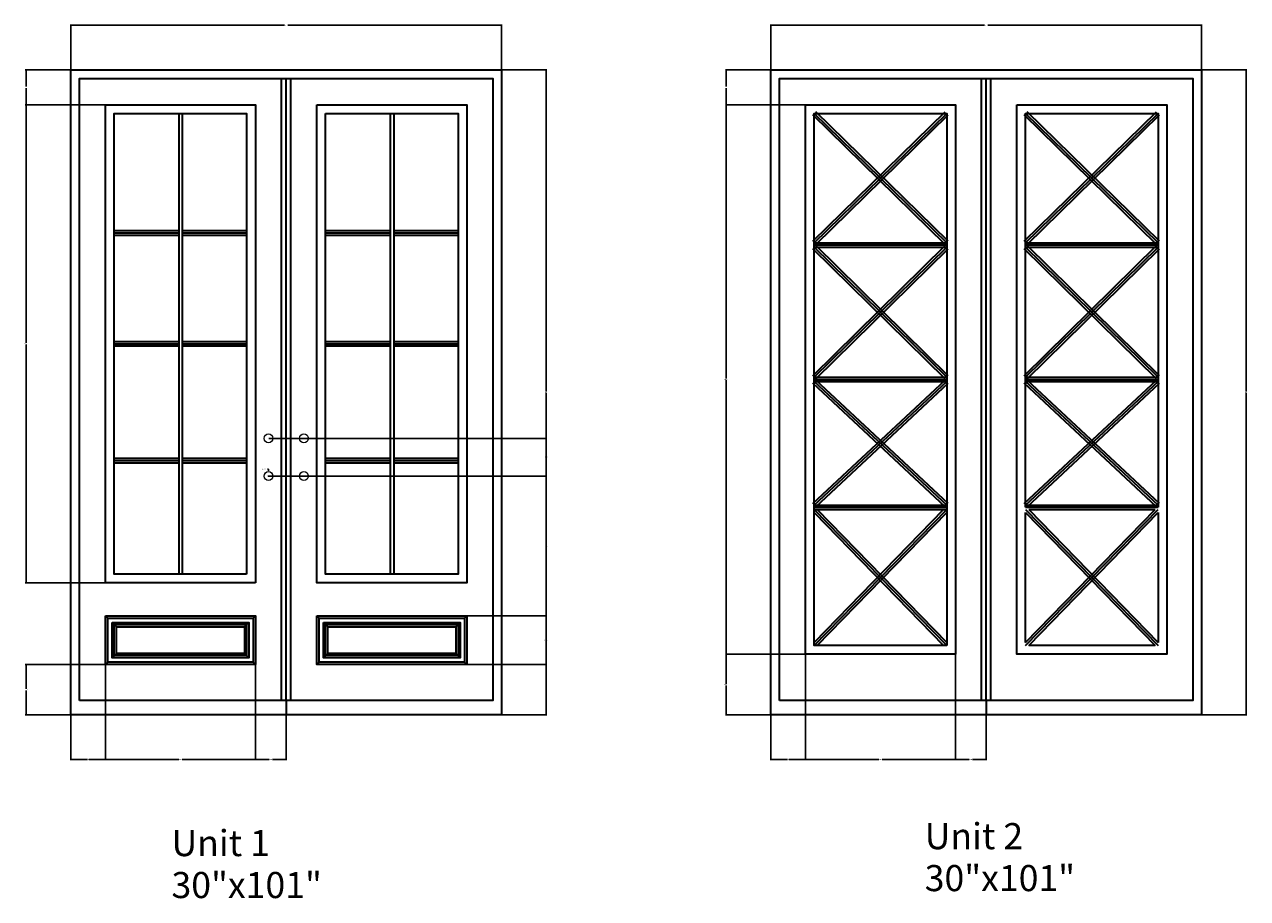
# Model space of a CAD drawing. Units: inches. Extents: x 1318 to 1980, y 617 to 1423.
# Tile 5 of 7: x 1351 to 1632, y 1222 to 1423. Entities that reach past the tile are written whole.
import ezdxf

# ---------------------------------------------------------------- set-up
doc = ezdxf.new("R2010")
doc.units = ezdxf.units.IN
doc.header["$MEASUREMENT"] = 0
for name, color, linetype, lineweight in [('A-ANNO-DIMS', 2, 'Continuous', 18), ('A-ANNO-TEXT', 7, 'Continuous', 25), ('A-DOOR', 4, 'Continuous', 35), ('A-DOOR-HDWR', 3, 'Continuous', 18)]:
    doc.layers.add(name, color=color, linetype=linetype, lineweight=lineweight)
doc.styles.get("Standard").update_dxf_attribs({"font": 'arial.ttf'})
doc.dimstyles.get("Standard").update_dxf_attribs({"dimtxt": 0.18, "dimasz": 0.18, "dimexe": 0.18, "dimexo": 0.0625, "dimgap": 0.09, "dimtad": 0, "dimtih": 1, "dimtoh": 1, "dimdec": 0, "dimzin": 0, "dimdsep": 46, "dimlunit": 3, "dimtxsty": 'Standard', "dimcen": 0.09, "dimadec": 0, "dimazin": 0, "dimtfac": 1, "dimtdec": 0, "dimtofl": 0, "dimtmove": 0, "dimatfit": 3, "dimfxl": 1, "dimtolj": 1, "dimtzin": 0, "dimarcsym": 0})

# ---------------------------------------------------------------- blocks, each defined once
blk = doc.blocks.new('DOOR-KNOB-SET')
for centre in [(1.01, 9.67), (9.16, 9.67), (1.01, 1.01), (9.16, 1.01)]:
    blk.add_circle(centre, 1.01)
blk = doc.blocks.new('*D4')
at = {"layer": 'A-ANNO-DIMS', "color": 0, "lineweight": -2, "transparency": 16777216}
for p, q in [((1453.13, 1287.17), (1471.5, 1287.17)), ((1471.32, 1286.99), (1471.32, 1281.77)), ((1471.32, 1276.2), (1471.32, 1281.41)), ((1453.13, 1276.02), (1471.5, 1276.02))]:
    blk.add_line(p, q, dxfattribs=at)
at = {"layer": 'A-ANNO-DIMS', "color": 0, "transparency": 16777216}
for points in [[(1471.29, 1286.99), (1471.35, 1286.99), (1471.32, 1287.17)], [(1471.29, 1276.2), (1471.35, 1276.2), (1471.32, 1276.02)]]:
    blk.add_solid(points, dxfattribs=at)
at = {"layer": 'Defpoints', "color": 0, "transparency": 16777216}
for p in [(1453.07, 1287.17), (1471.32, 1287.17), (1453.07, 1276.02)]:
    blk.add_point(p, dxfattribs=at)
at = {"layer": 'A-ANNO-DIMS', "color": 0, "transparency": 16777216, "insert": (1471.32, 1281.59), "char_height": 0.18, "attachment_point": 5}
blk.add_mtext('\\A1;11.142', dxfattribs=at)
blk = doc.blocks.new('*D5')
at = {"layer": 'A-ANNO-DIMS', "color": 0, "lineweight": -2, "transparency": 16777216}
for p, q in [((1407.58, 1319.29), (1471.5, 1319.29)), ((1471.32, 1319.11), (1471.32, 1303.41)), ((1471.32, 1287.35), (1471.32, 1303.04)), ((1453.13, 1287.17), (1471.5, 1287.17))]:
    blk.add_line(p, q, dxfattribs=at)
at = {"layer": 'A-ANNO-DIMS', "color": 0, "transparency": 16777216}
for points in [[(1471.29, 1319.11), (1471.35, 1319.11), (1471.32, 1319.29)], [(1471.29, 1287.35), (1471.35, 1287.35), (1471.32, 1287.17)]]:
    blk.add_solid(points, dxfattribs=at)
at = {"layer": 'Defpoints', "color": 0, "transparency": 16777216}
for p in [(1407.52, 1319.29), (1471.32, 1319.29), (1453.07, 1287.17)]:
    blk.add_point(p, dxfattribs=at)
at = {"layer": 'A-ANNO-DIMS', "color": 0, "transparency": 16777216, "insert": (1471.32, 1303.23), "char_height": 0.18, "attachment_point": 5}
blk.add_mtext('\\A1;32.12', dxfattribs=at)
blk = doc.blocks.new('*D6')
at = {"layer": 'A-ANNO-DIMS', "color": 0, "lineweight": -2, "transparency": 16777216}
for p, q in [((1407.58, 1327.95), (1471.5, 1327.95)), ((1471.32, 1327.77), (1471.32, 1323.8)), ((1471.32, 1319.47), (1471.32, 1323.44)), ((1407.58, 1319.29), (1471.5, 1319.29))]:
    blk.add_line(p, q, dxfattribs=at)
at = {"layer": 'A-ANNO-DIMS', "color": 0, "transparency": 16777216}
for points in [[(1471.29, 1327.77), (1471.35, 1327.77), (1471.32, 1327.95)], [(1471.29, 1319.47), (1471.35, 1319.47), (1471.32, 1319.29)]]:
    blk.add_solid(points, dxfattribs=at)
at = {"layer": 'Defpoints', "color": 0, "transparency": 16777216}
for p in [(1407.52, 1327.95), (1471.32, 1327.95), (1407.52, 1319.29)]:
    blk.add_point(p, dxfattribs=at)
at = {"layer": 'A-ANNO-DIMS', "color": 0, "transparency": 16777216, "insert": (1471.32, 1323.62), "char_height": 0.18, "attachment_point": 5}
blk.add_mtext('\\A1;8.663', dxfattribs=at)
blk = doc.blocks.new('*D7')
at = {"layer": 'A-ANNO-DIMS', "color": 0, "lineweight": -2, "transparency": 16777216}
for p, q in [((1362.09, 1412.68), (1362.09, 1423.04)), ((1362.27, 1422.86), (1411.18, 1422.86)), ((1460.89, 1422.86), (1411.97, 1422.86)), ((1461.07, 1412.68), (1461.07, 1423.04))]:
    blk.add_line(p, q, dxfattribs=at)
at = {"layer": 'A-ANNO-DIMS', "color": 0, "transparency": 16777216}
for points in [[(1362.27, 1422.89), (1362.27, 1422.83), (1362.09, 1422.86)], [(1460.89, 1422.89), (1460.89, 1422.83), (1461.07, 1422.86)]]:
    blk.add_solid(points, dxfattribs=at)
at = {"layer": 'Defpoints', "color": 0, "transparency": 16777216}
for p in [(1461.07, 1422.86), (1362.09, 1412.61), (1461.07, 1412.61)]:
    blk.add_point(p, dxfattribs=at)
at = {"layer": 'A-ANNO-DIMS', "color": 0, "transparency": 16777216, "insert": (1411.58, 1422.86), "char_height": 0.18, "attachment_point": 5}
blk.add_mtext('\\A1;98.98', dxfattribs=at)
blk = doc.blocks.new('*D8')
at = {"layer": 'A-ANNO-DIMS', "color": 0, "lineweight": -2, "transparency": 16777216}
for p, q in [((1461.13, 1412.61), (1471.5, 1412.61)), ((1471.32, 1412.43), (1471.32, 1338.7)), ((1471.32, 1264.59), (1471.32, 1338.33)), ((1461.13, 1264.41), (1471.5, 1264.41))]:
    blk.add_line(p, q, dxfattribs=at)
at = {"layer": 'A-ANNO-DIMS', "color": 0, "transparency": 16777216}
for points in [[(1471.29, 1412.43), (1471.35, 1412.43), (1471.32, 1412.61)], [(1471.29, 1264.59), (1471.35, 1264.59), (1471.32, 1264.41)]]:
    blk.add_solid(points, dxfattribs=at)
at = {"layer": 'Defpoints', "color": 0, "transparency": 16777216}
for p in [(1461.07, 1412.61), (1471.32, 1412.61), (1461.07, 1264.41)]:
    blk.add_point(p, dxfattribs=at)
at = {"layer": 'A-ANNO-DIMS', "color": 0, "transparency": 16777216, "insert": (1471.32, 1338.51), "char_height": 0.18, "attachment_point": 5}
blk.add_mtext('\\A1;148.2', dxfattribs=at)
blk = doc.blocks.new('*D9')
at = {"layer": 'A-ANNO-DIMS', "color": 0, "lineweight": -2, "transparency": 16777216}
for p, q in [((1370.09, 1275.96), (1370.09, 1253.98)), ((1362.09, 1264.35), (1362.09, 1253.98)), ((1362.27, 1254.16), (1365.94, 1254.16)), ((1369.91, 1254.16), (1366.24, 1254.16))]:
    blk.add_line(p, q, dxfattribs=at)
at = {"layer": 'A-ANNO-DIMS', "color": 0, "transparency": 16777216}
for points in [[(1362.27, 1254.19), (1362.27, 1254.13), (1362.09, 1254.16)], [(1369.91, 1254.19), (1369.91, 1254.13), (1370.09, 1254.16)]]:
    blk.add_solid(points, dxfattribs=at)
at = {"layer": 'Defpoints', "color": 0, "transparency": 16777216}
for p in [(1370.09, 1276.02), (1362.09, 1264.41), (1370.09, 1254.16)]:
    blk.add_point(p, dxfattribs=at)
at = {"layer": 'A-ANNO-DIMS', "color": 0, "transparency": 16777216, "insert": (1366.09, 1254.16), "char_height": 0.18, "attachment_point": 5}
blk.add_mtext('\\A1;8', dxfattribs=at)
blk = doc.blocks.new('*D10')
at = {"layer": 'A-ANNO-DIMS', "color": 0, "lineweight": -2, "transparency": 16777216}
for p, q in [((1370.09, 1275.96), (1370.09, 1253.98)), ((1404.51, 1275.96), (1404.51, 1253.98)), ((1370.27, 1254.16), (1386.91, 1254.16)), ((1404.33, 1254.16), (1387.69, 1254.16))]:
    blk.add_line(p, q, dxfattribs=at)
at = {"layer": 'A-ANNO-DIMS', "color": 0, "transparency": 16777216}
for points in [[(1370.27, 1254.19), (1370.27, 1254.13), (1370.09, 1254.16)], [(1404.33, 1254.19), (1404.33, 1254.13), (1404.51, 1254.16)]]:
    blk.add_solid(points, dxfattribs=at)
at = {"layer": 'Defpoints', "color": 0, "transparency": 16777216}
for p in [(1370.09, 1276.02), (1404.51, 1276.02), (1404.51, 1254.16)]:
    blk.add_point(p, dxfattribs=at)
at = {"layer": 'A-ANNO-DIMS', "color": 0, "transparency": 16777216, "insert": (1387.3, 1254.16), "char_height": 0.18, "attachment_point": 5}
blk.add_mtext('\\A1;34.42', dxfattribs=at)
blk = doc.blocks.new('*D11')
at = {"layer": 'A-ANNO-DIMS', "color": 0, "lineweight": -2, "transparency": 16777216}
for p, q in [((1404.51, 1275.96), (1404.51, 1253.98)), ((1411.58, 1264.35), (1411.58, 1253.98)), ((1404.69, 1254.16), (1407.65, 1254.16)), ((1411.4, 1254.16), (1408.44, 1254.16))]:
    blk.add_line(p, q, dxfattribs=at)
at = {"layer": 'A-ANNO-DIMS', "color": 0, "transparency": 16777216}
for points in [[(1404.69, 1254.19), (1404.69, 1254.13), (1404.51, 1254.16)], [(1411.4, 1254.19), (1411.4, 1254.13), (1411.58, 1254.16)]]:
    blk.add_solid(points, dxfattribs=at)
at = {"layer": 'Defpoints', "color": 0, "transparency": 16777216}
for p in [(1404.51, 1276.02), (1411.58, 1264.41), (1411.58, 1254.16)]:
    blk.add_point(p, dxfattribs=at)
at = {"layer": 'A-ANNO-DIMS', "color": 0, "transparency": 16777216, "insert": (1408.04, 1254.16), "char_height": 0.18, "attachment_point": 5}
blk.add_mtext('\\A1;7.068', dxfattribs=at)
blk = doc.blocks.new('*D12')
at = {"layer": 'A-ANNO-DIMS', "color": 0, "lineweight": -2, "transparency": 16777216}
for p, q in [((1370.02, 1276.02), (1351.66, 1276.02)), ((1351.84, 1275.84), (1351.84, 1270.4)), ((1351.84, 1264.59), (1351.84, 1270.04)), ((1362.02, 1264.41), (1351.66, 1264.41))]:
    blk.add_line(p, q, dxfattribs=at)
at = {"layer": 'A-ANNO-DIMS', "color": 0, "transparency": 16777216}
for points in [[(1351.81, 1275.84), (1351.87, 1275.84), (1351.84, 1276.02)], [(1351.81, 1264.59), (1351.87, 1264.59), (1351.84, 1264.41)]]:
    blk.add_solid(points, dxfattribs=at)
at = {"layer": 'Defpoints', "color": 0, "transparency": 16777216}
for p in [(1351.84, 1276.02), (1370.09, 1276.02), (1362.09, 1264.41)]:
    blk.add_point(p, dxfattribs=at)
at = {"layer": 'A-ANNO-DIMS', "color": 0, "transparency": 16777216, "insert": (1351.84, 1270.22), "char_height": 0.18, "attachment_point": 5}
blk.add_mtext('\\A1;11.61', dxfattribs=at)
blk = doc.blocks.new('*D13')
at = {"layer": 'A-ANNO-DIMS', "color": 0, "lineweight": -2, "transparency": 16777216}
for p, q in [((1370.02, 1404.61), (1351.66, 1404.61)), ((1351.84, 1404.43), (1351.84, 1349.86)), ((1351.84, 1294.93), (1351.84, 1349.5)), ((1370.02, 1294.75), (1351.66, 1294.75))]:
    blk.add_line(p, q, dxfattribs=at)
at = {"layer": 'A-ANNO-DIMS', "color": 0, "transparency": 16777216}
for points in [[(1351.81, 1404.43), (1351.87, 1404.43), (1351.84, 1404.61)], [(1351.81, 1294.93), (1351.87, 1294.93), (1351.84, 1294.75)]]:
    blk.add_solid(points, dxfattribs=at)
at = {"layer": 'Defpoints', "color": 0, "transparency": 16777216}
for p in [(1351.84, 1404.61), (1370.09, 1404.61), (1370.09, 1294.75)]:
    blk.add_point(p, dxfattribs=at)
at = {"layer": 'A-ANNO-DIMS', "color": 0, "transparency": 16777216, "insert": (1351.84, 1349.68), "char_height": 0.18, "attachment_point": 5}
blk.add_mtext('\\A1;109.87', dxfattribs=at)
blk = doc.blocks.new('*D14')
at = {"layer": 'A-ANNO-DIMS', "color": 0, "lineweight": -2, "transparency": 16777216}
for p, q in [((1362.02, 1412.61), (1351.66, 1412.61)), ((1351.84, 1412.43), (1351.84, 1408.8)), ((1351.84, 1404.79), (1351.84, 1408.43)), ((1370.02, 1404.61), (1351.66, 1404.61))]:
    blk.add_line(p, q, dxfattribs=at)
at = {"layer": 'A-ANNO-DIMS', "color": 0, "transparency": 16777216}
for points in [[(1351.81, 1412.43), (1351.87, 1412.43), (1351.84, 1412.61)], [(1351.81, 1404.79), (1351.87, 1404.79), (1351.84, 1404.61)]]:
    blk.add_solid(points, dxfattribs=at)
at = {"layer": 'Defpoints', "color": 0, "transparency": 16777216}
for p in [(1351.84, 1412.61), (1362.09, 1412.61), (1370.09, 1404.61)]:
    blk.add_point(p, dxfattribs=at)
at = {"layer": 'A-ANNO-DIMS', "color": 0, "transparency": 16777216, "insert": (1351.84, 1408.61), "char_height": 0.18, "attachment_point": 5}
blk.add_mtext('\\A1;8', dxfattribs=at)
blk = doc.blocks.new('*D15')
at = {"layer": 'A-ANNO-DIMS', "color": 0, "lineweight": -2, "transparency": 16777216}
for p, q in [((1522.91, 1412.68), (1522.91, 1423.04)), ((1523.09, 1422.86), (1572, 1422.86)), ((1621.7, 1422.86), (1572.79, 1422.86)), ((1621.88, 1412.68), (1621.88, 1423.04))]:
    blk.add_line(p, q, dxfattribs=at)
at = {"layer": 'A-ANNO-DIMS', "color": 0, "transparency": 16777216}
for points in [[(1523.09, 1422.89), (1523.09, 1422.83), (1522.91, 1422.86)], [(1621.7, 1422.89), (1621.7, 1422.83), (1621.88, 1422.86)]]:
    blk.add_solid(points, dxfattribs=at)
at = {"layer": 'Defpoints', "color": 0, "transparency": 16777216}
for p in [(1621.88, 1422.86), (1522.91, 1412.61), (1621.88, 1412.61)]:
    blk.add_point(p, dxfattribs=at)
at = {"layer": 'A-ANNO-DIMS', "color": 0, "transparency": 16777216, "insert": (1572.39, 1422.86), "char_height": 0.18, "attachment_point": 5}
blk.add_mtext('\\A1;98.98', dxfattribs=at)
blk = doc.blocks.new('*D16')
at = {"layer": 'A-ANNO-DIMS', "color": 0, "lineweight": -2, "transparency": 16777216}
for p, q in [((1621.95, 1412.61), (1632.31, 1412.61)), ((1632.13, 1412.43), (1632.13, 1338.7)), ((1632.13, 1264.59), (1632.13, 1338.33)), ((1621.95, 1264.41), (1632.31, 1264.41))]:
    blk.add_line(p, q, dxfattribs=at)
at = {"layer": 'A-ANNO-DIMS', "color": 0, "transparency": 16777216}
for points in [[(1632.1, 1412.43), (1632.16, 1412.43), (1632.13, 1412.61)], [(1632.1, 1264.59), (1632.16, 1264.59), (1632.13, 1264.41)]]:
    blk.add_solid(points, dxfattribs=at)
at = {"layer": 'Defpoints', "color": 0, "transparency": 16777216}
for p in [(1621.88, 1412.61), (1632.13, 1412.61), (1621.88, 1264.41)]:
    blk.add_point(p, dxfattribs=at)
at = {"layer": 'A-ANNO-DIMS', "color": 0, "transparency": 16777216, "insert": (1632.13, 1338.51), "char_height": 0.18, "attachment_point": 5}
blk.add_mtext('\\A1;148.2', dxfattribs=at)
blk = doc.blocks.new('*D17')
at = {"layer": 'A-ANNO-DIMS', "color": 0, "lineweight": -2, "transparency": 16777216}
for p, q in [((1530.91, 1278.29), (1530.91, 1253.98)), ((1522.91, 1264.35), (1522.91, 1253.98)), ((1523.09, 1254.16), (1526.76, 1254.16)), ((1530.73, 1254.16), (1527.05, 1254.16))]:
    blk.add_line(p, q, dxfattribs=at)
at = {"layer": 'A-ANNO-DIMS', "color": 0, "transparency": 16777216}
for points in [[(1523.09, 1254.19), (1523.09, 1254.13), (1522.91, 1254.16)], [(1530.73, 1254.19), (1530.73, 1254.13), (1530.91, 1254.16)]]:
    blk.add_solid(points, dxfattribs=at)
at = {"layer": 'Defpoints', "color": 0, "transparency": 16777216}
for p in [(1530.91, 1278.35), (1522.91, 1264.41), (1530.91, 1254.16)]:
    blk.add_point(p, dxfattribs=at)
at = {"layer": 'A-ANNO-DIMS', "color": 0, "transparency": 16777216, "insert": (1526.91, 1254.16), "char_height": 0.18, "attachment_point": 5}
blk.add_mtext('\\A1;8', dxfattribs=at)
blk = doc.blocks.new('*D18')
at = {"layer": 'A-ANNO-DIMS', "color": 0, "lineweight": -2, "transparency": 16777216}
for p, q in [((1530.91, 1278.29), (1530.91, 1253.98)), ((1565.33, 1278.29), (1565.33, 1253.98)), ((1531.09, 1254.16), (1547.72, 1254.16)), ((1565.15, 1254.16), (1548.51, 1254.16))]:
    blk.add_line(p, q, dxfattribs=at)
at = {"layer": 'A-ANNO-DIMS', "color": 0, "transparency": 16777216}
for points in [[(1531.09, 1254.19), (1531.09, 1254.13), (1530.91, 1254.16)], [(1565.15, 1254.19), (1565.15, 1254.13), (1565.33, 1254.16)]]:
    blk.add_solid(points, dxfattribs=at)
at = {"layer": 'Defpoints', "color": 0, "transparency": 16777216}
for p in [(1530.91, 1278.35), (1565.33, 1278.35), (1565.33, 1254.16)]:
    blk.add_point(p, dxfattribs=at)
at = {"layer": 'A-ANNO-DIMS', "color": 0, "transparency": 16777216, "insert": (1548.12, 1254.16), "char_height": 0.18, "attachment_point": 5}
blk.add_mtext('\\A1;34.42', dxfattribs=at)
blk = doc.blocks.new('*D19')
at = {"layer": 'A-ANNO-DIMS', "color": 0, "lineweight": -2, "transparency": 16777216}
for p, q in [((1565.33, 1278.29), (1565.33, 1253.98)), ((1572.39, 1264.35), (1572.39, 1253.98)), ((1565.51, 1254.16), (1568.47, 1254.16)), ((1572.21, 1254.16), (1569.25, 1254.16))]:
    blk.add_line(p, q, dxfattribs=at)
at = {"layer": 'A-ANNO-DIMS', "color": 0, "transparency": 16777216}
for points in [[(1565.51, 1254.19), (1565.51, 1254.13), (1565.33, 1254.16)], [(1572.21, 1254.19), (1572.21, 1254.13), (1572.39, 1254.16)]]:
    blk.add_solid(points, dxfattribs=at)
at = {"layer": 'Defpoints', "color": 0, "transparency": 16777216}
for p in [(1565.33, 1278.35), (1572.39, 1264.41), (1572.39, 1254.16)]:
    blk.add_point(p, dxfattribs=at)
at = {"layer": 'A-ANNO-DIMS', "color": 0, "transparency": 16777216, "insert": (1568.86, 1254.16), "char_height": 0.18, "attachment_point": 5}
blk.add_mtext('\\A1;7.068', dxfattribs=at)
blk = doc.blocks.new('*D20')
at = {"layer": 'A-ANNO-DIMS', "color": 0, "lineweight": -2, "transparency": 16777216}
for p, q in [((1530.84, 1278.35), (1512.48, 1278.35)), ((1512.66, 1278.17), (1512.66, 1271.56)), ((1512.66, 1264.59), (1512.66, 1271.2)), ((1522.84, 1264.41), (1512.48, 1264.41))]:
    blk.add_line(p, q, dxfattribs=at)
at = {"layer": 'A-ANNO-DIMS', "color": 0, "transparency": 16777216}
for points in [[(1512.63, 1278.17), (1512.69, 1278.17), (1512.66, 1278.35)], [(1512.63, 1264.59), (1512.69, 1264.59), (1512.66, 1264.41)]]:
    blk.add_solid(points, dxfattribs=at)
at = {"layer": 'Defpoints', "color": 0, "transparency": 16777216}
for p in [(1512.66, 1278.35), (1530.91, 1278.35), (1522.91, 1264.41)]:
    blk.add_point(p, dxfattribs=at)
at = {"layer": 'A-ANNO-DIMS', "color": 0, "transparency": 16777216, "insert": (1512.66, 1271.38), "char_height": 0.18, "attachment_point": 5}
blk.add_mtext('\\A1;13.939', dxfattribs=at)
blk = doc.blocks.new('*D21')
at = {"layer": 'A-ANNO-DIMS', "color": 0, "lineweight": -2, "transparency": 16777216}
for p, q in [((1530.84, 1404.61), (1512.48, 1404.61)), ((1512.66, 1404.43), (1512.66, 1341.67)), ((1512.66, 1278.53), (1512.66, 1341.3)), ((1530.84, 1278.35), (1512.48, 1278.35))]:
    blk.add_line(p, q, dxfattribs=at)
at = {"layer": 'A-ANNO-DIMS', "color": 0, "transparency": 16777216}
for points in [[(1512.63, 1404.43), (1512.69, 1404.43), (1512.66, 1404.61)], [(1512.63, 1278.53), (1512.69, 1278.53), (1512.66, 1278.35)]]:
    blk.add_solid(points, dxfattribs=at)
at = {"layer": 'Defpoints', "color": 0, "transparency": 16777216}
for p in [(1512.66, 1404.61), (1530.91, 1404.61), (1530.91, 1278.35)]:
    blk.add_point(p, dxfattribs=at)
at = {"layer": 'A-ANNO-DIMS', "color": 0, "transparency": 16777216, "insert": (1512.66, 1341.48), "char_height": 0.18, "attachment_point": 5}
blk.add_mtext('\\A1;126.26', dxfattribs=at)
blk = doc.blocks.new('*D22')
at = {"layer": 'A-ANNO-DIMS', "color": 0, "lineweight": -2, "transparency": 16777216}
for p, q in [((1522.84, 1412.61), (1512.48, 1412.61)), ((1512.66, 1412.43), (1512.66, 1408.8)), ((1512.66, 1404.79), (1512.66, 1408.43)), ((1530.84, 1404.61), (1512.48, 1404.61))]:
    blk.add_line(p, q, dxfattribs=at)
at = {"layer": 'A-ANNO-DIMS', "color": 0, "transparency": 16777216}
for points in [[(1512.63, 1412.43), (1512.69, 1412.43), (1512.66, 1412.61)], [(1512.63, 1404.79), (1512.69, 1404.79), (1512.66, 1404.61)]]:
    blk.add_solid(points, dxfattribs=at)
at = {"layer": 'Defpoints', "color": 0, "transparency": 16777216}
for p in [(1512.66, 1412.61), (1522.91, 1412.61), (1530.91, 1404.61)]:
    blk.add_point(p, dxfattribs=at)
at = {"layer": 'A-ANNO-DIMS', "color": 0, "transparency": 16777216, "insert": (1512.66, 1408.61), "char_height": 0.18, "attachment_point": 5}
blk.add_mtext('\\A1;8', dxfattribs=at)
blk = doc.blocks.new('*D104')
at = {"layer": 'A-ANNO-DIMS', "color": 0, "lineweight": -2, "transparency": 16777216}
for p, q in [((1407.31, 1320.9), (1407.49, 1320.9)), ((1407.49, 1320.9), (1407.5, 1320.47)), ((1407.43, 1319.29), (1407.61, 1319.29)), ((1407.52, 1319.2), (1407.52, 1319.38))]:
    blk.add_line(p, q, dxfattribs=at)
at = {"layer": 'A-ANNO-DIMS', "color": 0, "transparency": 16777216}
blk.add_solid([(1407.53, 1320.48), (1407.47, 1320.47), (1407.5, 1320.29)], dxfattribs=at)
at = {"layer": 'Defpoints', "color": 0, "transparency": 16777216}
for p in [(1407.5, 1320.29), (1407.53, 1318.28)]:
    blk.add_point(p, dxfattribs=at)
at = {"layer": 'A-ANNO-DIMS', "color": 0, "transparency": 16777216, "insert": (1406.63, 1320.9), "char_height": 0.18, "attachment_point": 5}
blk.add_mtext('\\A1;4X ∅2.017', dxfattribs=at)

msp = doc.modelspace()

# ---------------------------------------------------------------- linework, layer by layer
at = {"layer": 'A-DOOR'}
for p, q in [((1410.5087, 1267.7069), (1410.5087, 1410.615)), ((1411.5767, 1267.7069), (1411.5767, 1410.615)), ((1412.6446, 1267.7069), (1412.6446, 1410.615)), ((1571.3268, 1267.7069), (1571.3268, 1410.615)), ((1572.3947, 1267.7069), (1572.3947, 1410.615)), ((1573.4627, 1267.7069), (1573.4627, 1410.615)), ((1386.9042, 1402.615), (1386.9042, 1296.7497)), ((1387.7277, 1402.615), (1387.7277, 1296.7497)), ((1435.4614, 1402.615), (1435.4614, 1296.7497)), ((1436.2849, 1402.615), (1436.2849, 1296.7497)), ((1532.556, 1373.2363), (1562.9773, 1402.9725)), ((1562.9773, 1372.5212), (1532.556, 1402.2574)), ((1532.9055, 1372.8787), (1563.3268, 1402.615)), ((1563.3268, 1372.8787), (1532.9055, 1402.615)), ((1563.6763, 1373.2363), (1533.255, 1402.9725)), ((1533.255, 1372.5212), (1563.6763, 1402.2574)), ((1581.1132, 1373.2363), (1611.5345, 1402.9725)), ((1611.5345, 1372.5212), (1581.1132, 1402.2574)), ((1581.4627, 1372.8787), (1611.884, 1402.615)), ((1611.884, 1372.8787), (1581.4627, 1402.615)), ((1612.2335, 1373.2363), (1581.8122, 1402.9725)), ((1581.8122, 1372.5212), (1612.2335, 1402.2574)), ((1372.0874, 1375.6684), (1386.9042, 1375.6684)), ((1372.0874, 1375.1684), (1386.9042, 1375.1684)), ((1372.0874, 1374.6684), (1386.9042, 1374.6684)), ((1387.7277, 1375.6684), (1402.5087, 1375.6684)), ((1387.7277, 1375.1684), (1402.5087, 1375.1684)), ((1387.7277, 1374.6684), (1402.5087, 1374.6684)), ((1420.6446, 1375.6684), (1435.4614, 1375.6684)), ((1420.6446, 1375.1684), (1435.4614, 1375.1684)), ((1420.6446, 1374.6684), (1435.4614, 1374.6684)), ((1436.2849, 1375.6684), (1451.0659, 1375.6684)), ((1436.2849, 1375.1684), (1451.0659, 1375.1684)), ((1436.2849, 1374.6684), (1451.0659, 1374.6684)), ((1532.555, 1342.3402), (1562.9763, 1372.2354)), ((1562.9763, 1341.6269), (1532.555, 1371.5221)), ((1532.9055, 1372.8787), (1563.3268, 1372.8787)), ((1532.9055, 1372.3787), (1563.3268, 1372.3787)), ((1532.9055, 1371.8787), (1563.3268, 1371.8787)), ((1532.9055, 1341.9835), (1563.3268, 1371.8787)), ((1563.3268, 1341.9835), (1532.9055, 1371.8787)), ((1563.6772, 1342.3402), (1533.256, 1372.2354)), ((1533.256, 1341.6269), (1563.6772, 1371.5221)), ((1581.1122, 1342.3402), (1611.5335, 1372.2354)), ((1611.5335, 1341.6269), (1581.1122, 1371.5221)), ((1581.4627, 1372.8787), (1611.884, 1372.8787)), ((1581.4627, 1372.3787), (1611.884, 1372.3787)), ((1581.4627, 1371.8787), (1611.884, 1371.8787)), ((1581.4627, 1341.9835), (1611.884, 1371.8787)), ((1611.884, 1341.9835), (1581.4627, 1371.8787)), ((1612.2344, 1342.3402), (1581.8132, 1372.2354)), ((1581.8132, 1341.6269), (1612.2344, 1371.5221)), ((1372.0874, 1350.1824), (1386.9042, 1350.1824)), ((1372.0874, 1349.6824), (1386.9042, 1349.6824)), ((1372.0874, 1349.1824), (1386.9042, 1349.1824)), ((1387.7277, 1350.1824), (1402.5087, 1350.1824)), ((1387.7277, 1349.6824), (1402.5087, 1349.6824)), ((1387.7277, 1349.1824), (1402.5087, 1349.1824)), ((1420.6446, 1350.1824), (1435.4614, 1350.1824)), ((1420.6446, 1349.6824), (1435.4614, 1349.6824)), ((1420.6446, 1349.1824), (1435.4614, 1349.1824)), ((1436.2849, 1350.1824), (1451.0659, 1350.1824)), ((1436.2849, 1349.6824), (1451.0659, 1349.6824)), ((1436.2849, 1349.1824), (1451.0659, 1349.1824)), ((1532.5645, 1312.9808), (1562.9858, 1341.3492)), ((1562.9858, 1312.2494), (1532.5645, 1340.6179)), ((1532.9055, 1341.9835), (1563.3268, 1341.9835)), ((1532.9055, 1341.4835), (1563.3268, 1341.4835)), ((1532.9055, 1340.9835), (1563.3268, 1340.9835)), ((1532.9055, 1312.6151), (1563.3268, 1340.9835)), ((1563.3268, 1312.6151), (1532.9055, 1340.9835)), ((1563.6678, 1312.9808), (1533.2465, 1341.3492)), ((1533.2465, 1312.2494), (1563.6678, 1340.6179)), ((1581.1217, 1312.9808), (1611.543, 1341.3492)), ((1611.543, 1312.2494), (1581.1217, 1340.6179)), ((1581.4627, 1341.9835), (1611.884, 1341.9835)), ((1581.4627, 1341.4835), (1611.884, 1341.4835)), ((1581.4627, 1340.9835), (1611.884, 1340.9835)), ((1581.4627, 1312.6151), (1611.884, 1340.9835)), ((1611.884, 1312.6151), (1581.4627, 1340.9835)), ((1612.225, 1312.9808), (1581.8037, 1341.3492)), ((1581.8037, 1312.2494), (1612.225, 1340.6179)), ((1372.0874, 1323.3594), (1386.9042, 1323.3594)), ((1372.0874, 1322.8594), (1386.9042, 1322.8594)), ((1372.0874, 1322.3594), (1386.9042, 1322.3594)), ((1387.7277, 1323.3594), (1402.5087, 1323.3594)), ((1387.7277, 1322.8594), (1402.5087, 1322.8594)), ((1387.7277, 1322.3594), (1402.5087, 1322.3594)), ((1420.6446, 1323.3594), (1435.4614, 1323.3594)), ((1420.6446, 1322.8594), (1435.4614, 1322.8594)), ((1420.6446, 1322.3594), (1435.4614, 1322.3594)), ((1436.2849, 1323.3594), (1451.0659, 1323.3594)), ((1436.2849, 1322.8594), (1451.0659, 1322.8594)), ((1436.2849, 1322.3594), (1451.0659, 1322.3594)), ((1532.9055, 1312.6151), (1563.3268, 1312.6151)), ((1581.4627, 1312.6151), (1611.884, 1312.6151)), ((1532.9055, 1312.1151), (1563.3268, 1312.1151)), ((1532.9055, 1311.6151), (1563.3268, 1311.6151)), ((1532.9055, 1280.3521), (1563.3268, 1311.6151)), ((1563.3268, 1280.3521), (1532.9055, 1311.6151)), ((1532.9055, 1281.0691), (1562.6291, 1311.6151)), ((1532.9055, 1310.8982), (1562.6291, 1280.3521)), ((1533.6031, 1311.6151), (1562.6291, 1311.6151)), ((1533.6031, 1311.6151), (1563.3268, 1281.0691)), ((1533.6031, 1280.3521), (1563.3268, 1310.8982)), ((1581.4627, 1312.1151), (1611.884, 1312.1151)), ((1581.4627, 1280.3521), (1611.884, 1311.6151)), ((1581.4627, 1311.6151), (1611.884, 1280.3521)), ((1581.4627, 1281.0691), (1611.1863, 1311.6151)), ((1581.4627, 1310.8982), (1611.1863, 1280.3521)), ((1582.1604, 1311.6151), (1611.1863, 1311.6151)), ((1582.1604, 1311.6151), (1611.884, 1281.0691)), ((1582.1604, 1280.3521), (1611.884, 1310.8982)), ((1370.0874, 1287.1657), (1370.5874, 1286.6657)), ((1404.0087, 1286.6657), (1404.5087, 1287.1657)), ((1418.6446, 1287.1657), (1419.1446, 1286.6657)), ((1452.5659, 1286.6657), (1453.0659, 1287.1657)), ((1371.5874, 1285.6657), (1372.5874, 1284.6657)), ((1402.0087, 1284.6657), (1403.0087, 1285.6657)), ((1420.1446, 1285.6657), (1421.1446, 1284.6657)), ((1450.5659, 1284.6657), (1451.5659, 1285.6657)), ((1371.5874, 1277.5233), (1372.5874, 1278.5233)), ((1403.0087, 1277.5233), (1402.0087, 1278.5233)), ((1420.1446, 1277.5233), (1421.1446, 1278.5233)), ((1451.5659, 1277.5233), (1450.5659, 1278.5233)), ((1370.0874, 1276.0233), (1370.5874, 1276.5233)), ((1404.5087, 1276.0233), (1404.0087, 1276.5233)), ((1418.6446, 1276.0233), (1419.1446, 1276.5233)), ((1453.0659, 1276.0233), (1452.5659, 1276.5233)), ((1411.5767, 1267.7069), (1411.5767, 1264.4136)), ((1572.3947, 1267.7069), (1572.3947, 1264.4136))]:
    msp.add_line(p, q, dxfattribs=at)
for points in [[(1362.0874, 1412.615), (1461.0659, 1412.615), (1461.0659, 1264.4136), (1362.0874, 1264.4136)], [(1364.0874, 1267.7069), (1364.0874, 1410.615), (1459.0659, 1410.615), (1459.0659, 1267.7069)], [(1522.9055, 1412.615), (1621.884, 1412.615), (1621.884, 1264.4136), (1522.9055, 1264.4136)], [(1524.9055, 1267.7069), (1524.9055, 1410.615), (1619.884, 1410.615), (1619.884, 1267.7069)], [(1404.5087, 1294.7497), (1370.0874, 1294.7497), (1370.0874, 1404.615), (1404.5087, 1404.615)], [(1402.5087, 1296.7497), (1372.0874, 1296.7497), (1372.0874, 1402.615), (1402.5087, 1402.615)], [(1418.6446, 1404.615), (1453.0659, 1404.615), (1453.0659, 1294.7497), (1418.6446, 1294.7497)], [(1420.6446, 1402.615), (1451.0659, 1402.615), (1451.0659, 1296.7497), (1420.6446, 1296.7497)], [(1565.3268, 1278.3521), (1530.9055, 1278.3521), (1530.9055, 1404.615), (1565.3268, 1404.615)], [(1563.3268, 1280.3521), (1532.9055, 1280.3521), (1532.9055, 1402.615), (1563.3268, 1402.615)], [(1579.4627, 1404.615), (1613.884, 1404.615), (1613.884, 1278.3521), (1579.4627, 1278.3521)], [(1370.0874, 1287.1657), (1404.5087, 1287.1657), (1404.5087, 1276.0233), (1370.0874, 1276.0233)], [(1418.6446, 1287.1657), (1453.0659, 1287.1657), (1453.0659, 1276.0233), (1418.6446, 1276.0233)], [(1370.5874, 1286.6657), (1404.0087, 1286.6657), (1404.0087, 1276.5233), (1370.5874, 1276.5233)], [(1371.5874, 1285.6657), (1403.0087, 1285.6657), (1403.0087, 1277.5233), (1371.5874, 1277.5233)], [(1372.0874, 1285.1657), (1402.5087, 1285.1657), (1402.5087, 1278.0233), (1372.0874, 1278.0233)], [(1372.5874, 1284.6657), (1402.0087, 1284.6657), (1402.0087, 1278.5233), (1372.5874, 1278.5233)], [(1419.1446, 1286.6657), (1452.5659, 1286.6657), (1452.5659, 1276.5233), (1419.1446, 1276.5233)], [(1420.1446, 1285.6657), (1451.5659, 1285.6657), (1451.5659, 1277.5233), (1420.1446, 1277.5233)], [(1420.6446, 1285.1657), (1451.0659, 1285.1657), (1451.0659, 1278.0233), (1420.6446, 1278.0233)], [(1421.1446, 1284.6657), (1450.5659, 1284.6657), (1450.5659, 1278.5233), (1421.1446, 1278.5233)]]:
    msp.add_lwpolyline(points, close=True, dxfattribs=at)
for points in [[(1581.4627, 1312.1151), (1581.4627, 1402.615), (1611.884, 1402.615), (1611.884, 1312.1151)], [(1532.9055, 1281.0691), (1532.9055, 1310.8982)], [(1563.3268, 1310.8982), (1563.3268, 1281.0691)], [(1581.4627, 1281.0691), (1581.4627, 1310.8982)], [(1611.884, 1310.8982), (1611.884, 1281.0691)], [(1562.6291, 1280.3521), (1533.6031, 1280.3521)], [(1611.1863, 1280.3521), (1582.1604, 1280.3521)]]:
    msp.add_lwpolyline(points, dxfattribs=at)

# ---------------------------------------------------------------- block references
at = {"layer": 'A-DOOR-HDWR'}
msp.add_blockref('DOOR-KNOB-SET', (1406.507, 1318.278), dxfattribs=at)

# ---------------------------------------------------------------- texts
at = {"layer": 'A-ANNO-TEXT'}
for s, p in [('Unit 2', (1558.2748, 1233.5526)), ('Unit 1', (1385.2363, 1231.9597)), ('30"x101"', (1385.2363, 1222.3213)), ('30"x101"', (1558.2748, 1223.9142))]:
    msp.add_text(s, height=6, dxfattribs=at).set_placement(p)

# ---------------------------------------------------------------- dimensions: what is measured, and where the dimension line sits
at = {"layer": 'A-ANNO-DIMS'}
for base, p1, p2, override, picture, middle in [((1461.0659, 1422.865), (1362.0874, 1412.615), (1461.0659, 1412.615), {"dimdec": 2, "dimlfac": 1, "dimrnd": 0, "dimzin": 0, "dimdsep": 46, "dimlunit": 2}, '*D7', (1411.5767, 1422.865)), ((1621.884, 1422.865), (1522.9055, 1412.615), (1621.884, 1412.615), {"dimdec": 2, "dimlfac": 1, "dimrnd": 0, "dimzin": 0, "dimdsep": 46, "dimlunit": 2}, '*D15', (1572.3947, 1422.865)), ((1370.0874, 1254.1636), (1362.0874, 1264.4136), (1370.0874, 1276.0233), {"dimdec": 0, "dimlfac": 1, "dimrnd": 0, "dimzin": 0, "dimdsep": 46, "dimlunit": 2}, '*D9', (1366.0874, 1254.1636)), ((1404.5087, 1254.1636), (1370.0874, 1276.0233), (1404.5087, 1276.0233), {"dimdec": 2, "dimlfac": 1, "dimrnd": 0, "dimzin": 0, "dimdsep": 46, "dimlunit": 2}, '*D10', (1387.2981, 1254.1636)), ((1411.5767, 1254.1636), (1404.5087, 1276.0233), (1411.5767, 1264.4136), {"dimdec": 3, "dimlfac": 1, "dimrnd": 0, "dimzin": 0, "dimdsep": 46, "dimlunit": 2}, '*D11', (1408.0427, 1254.1636)), ((1530.9055, 1254.1636), (1522.9055, 1264.4136), (1530.9055, 1278.3521), {"dimdec": 0, "dimlfac": 1, "dimrnd": 0, "dimzin": 0, "dimdsep": 46, "dimlunit": 2}, '*D17', (1526.9055, 1254.1636)), ((1565.3268, 1254.1636), (1530.9055, 1278.3521), (1565.3268, 1278.3521), {"dimdec": 2, "dimlfac": 1, "dimrnd": 0, "dimzin": 0, "dimdsep": 46, "dimlunit": 2}, '*D18', (1548.1161, 1254.1636)), ((1572.3947, 1254.1636), (1565.3268, 1278.3521), (1572.3947, 1264.4136), {"dimdec": 3, "dimlfac": 1, "dimrnd": 0, "dimzin": 0, "dimdsep": 46, "dimlunit": 2}, '*D19', (1568.8608, 1254.1636))]:
    dim = msp.add_linear_dim(base=base, p1=p1, p2=p2, dimstyle='Standard', override=override, dxfattribs=at)
    dim.commit()
    dim.dimension.update_dxf_attribs({"geometry": picture, "text_midpoint": middle})
for base, p1, p2, override, picture, middle in [((1351.8374, 1412.615), (1370.0874, 1404.615), (1362.0874, 1412.615), {"dimdec": 0, "dimlfac": 1, "dimrnd": 0, "dimzin": 0, "dimdsep": 46, "dimlunit": 2}, '*D14', (1351.8374, 1408.615)), ((1471.3159, 1412.615), (1461.0659, 1264.4136), (1461.0659, 1412.615), {"dimdec": 1, "dimlfac": 1, "dimrnd": 0, "dimzin": 0, "dimdsep": 46, "dimlunit": 2}, '*D8', (1471.3159, 1338.5143)), ((1512.6555, 1412.615), (1530.9055, 1404.615), (1522.9055, 1412.615), {"dimdec": 0, "dimlfac": 1, "dimrnd": 0, "dimzin": 0, "dimdsep": 46, "dimlunit": 2}, '*D22', (1512.6555, 1408.615)), ((1632.134, 1412.615), (1621.884, 1264.4136), (1621.884, 1412.615), {"dimdec": 1, "dimlfac": 1, "dimrnd": 0, "dimzin": 0, "dimdsep": 46, "dimlunit": 2}, '*D16', (1632.134, 1338.5143)), ((1351.8374, 1404.615), (1370.0874, 1294.7497), (1370.0874, 1404.615), {"dimdec": 2, "dimlfac": 1, "dimrnd": 0, "dimzin": 0, "dimdsep": 46, "dimlunit": 2}, '*D13', (1351.8374, 1349.6824)), ((1512.6555, 1404.615), (1530.9055, 1278.3521), (1530.9055, 1404.615), {"dimdec": 2, "dimlfac": 1, "dimrnd": 0, "dimzin": 0, "dimdsep": 46, "dimlunit": 2}, '*D21', (1512.6555, 1341.4835)), ((1471.3159, 1327.9494), (1407.516, 1319.2865), (1407.516, 1327.9494), {"dimdec": 3, "dimlfac": 1, "dimrnd": 0, "dimzin": 0, "dimdsep": 46, "dimlunit": 2}, '*D6', (1471.3159, 1323.618)), ((1471.3159, 1319.2865), (1453.0659, 1287.1657), (1407.516, 1319.2865), {"dimdec": 2, "dimlfac": 1, "dimrnd": 0, "dimzin": 0, "dimdsep": 46, "dimlunit": 2}, '*D5', (1471.3159, 1303.2261)), ((1471.3159, 1287.1657), (1453.0659, 1276.0233), (1453.0659, 1287.1657), {"dimdec": 3, "dimlfac": 1, "dimrnd": 0, "dimzin": 0, "dimdsep": 46, "dimlunit": 2}, '*D4', (1471.3159, 1281.5945)), ((1351.8374, 1276.0233), (1362.0874, 1264.4136), (1370.0874, 1276.0233), {"dimdec": 2, "dimlfac": 1, "dimrnd": 0, "dimzin": 0, "dimdsep": 46, "dimlunit": 2}, '*D12', (1351.8374, 1270.2184)), ((1512.6555, 1278.3521), (1522.9055, 1264.41359), (1530.9055, 1278.3521), {"dimdec": 3, "dimlfac": 1, "dimrnd": 0, "dimzin": 0, "dimdsep": 46, "dimlunit": 2}, '*D20', (1512.6555, 1271.38285))]:
    dim = msp.add_linear_dim(base=base, p1=p1, p2=p2, angle=90, dimstyle='Standard', override=override, dxfattribs=at)
    dim.commit()
    dim.dimension.update_dxf_attribs({"geometry": picture, "text_midpoint": middle})
dim = msp.add_diameter_dim_2p(p1=(1407.5319, 1318.2781), p2=(1407.5001, 1320.2949), text='4X <>', dimstyle='Standard', override={"dimdec": 3, "dimlfac": 1, "dimrnd": 0, "dimzin": 0, "dimdsep": 46, "dimlunit": 2}, dxfattribs=at)
dim.commit()
dim.dimension.update_dxf_attribs({"geometry": '*D104', "text_midpoint": (1406.6267, 1320.9), "dimtype": 163})

doc.saveas('drawing.dxf')
